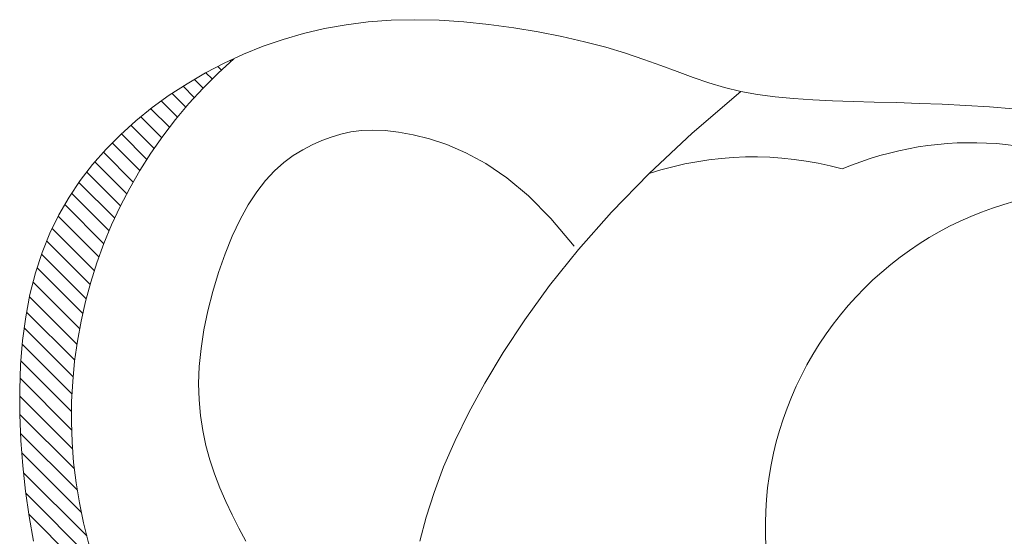
# Model space of a CAD drawing. Units: inches. Extents: x -17 to 1735, y -531 to 60.
# Tile 8 of 27: x 1734.671706 to 1734.675388, y -150.218274 to -150.216342. Entities that reach past the tile are written whole.
import ezdxf

# ---------------------------------------------------------------- set-up
doc = ezdxf.new("R2010")
doc.units = ezdxf.units.IN
doc.header["$MEASUREMENT"] = 0
doc.layers.add('A-FURN', color=242, linetype='Continuous', lineweight=18, true_color=0xcd2027)

# ---------------------------------------------------------------- blocks, each defined once
blk = doc.blocks.new('childrens_room_2')
for p, q in [((70.11022739858484, 54.15762691826097), (70.11227292050492, 54.15799201522753)), ((70.11227292050492, 54.15799201522753), (70.11437812355464, 54.15825517993511)), ((70.11437812355464, 54.15825517993511), (70.11654878333096, 54.1584144891371)), ((70.11654878333096, 54.1584144891371), (70.1187906754308, 54.15846801959418)), ((70.1187906754308, 54.15846801959418), (70.12110363943387, 54.15841577130635)), ((70.12110363943387, 54.15841577130635), (70.1234637707926, 54.15826543726729)), ((70.1234637707926, 54.15826543726729), (70.12584122900037, 54.15802663372454)), ((70.12584122900037, 54.15802663372454), (70.12820617337594, 54.15770897692567)), ((70.10629229580402, 54.15659862055185), (70.10823578225566, 54.1571618122893)), ((70.10823578225566, 54.1571618122893), (70.11022739858484, 54.15762691826097)), ((70.12820617337594, 54.15770897692567), (70.13052876347095, 54.15732208312551)), ((70.13052876347095, 54.15732208312551), (70.13277915866232, 54.15687556855704)), ((70.13277915866232, 54.15687556855704), (70.13492751844345, 54.15637904946783)), ((70.10252661037842, 54.15518567278053), (70.10439116369119, 54.15593926630248)), ((70.10439116369119, 54.15593926630248), (70.10629229580402, 54.15659862055185)), ((70.13492751844345, 54.15637904946783), (70.13694400219131, 54.15584214210543)), ((70.10069526663167, 54.15434008377491), (70.10252661037842, 54.15518567278053)), ((70.13694400219131, 54.15584214210543), (70.13880855579512, 54.1552752640768)), ((70.13880855579512, 54.1552752640768), (70.14054027072737, 54.15469203840479)), ((70.09890338942526, 54.15340602525105), (70.10069526663167, 54.15434008377491)), ((70.10042017687695, 54.15368526775131), (70.10008399876418, 54.15402144587864)), ((70.10132402636694, 54.15451022646306), (70.1012418118876, 54.15459244092057)), ((70.14054027072737, 54.15469203840479), (70.14216802503098, 54.15410688947162)), ((70.14216802503098, 54.15410688947162), (70.14372069663251, 54.15353424165227)), ((70.0971596421546, 54.15238734370217), (70.09890338942526, 54.15340602525105)), ((70.09953980340973, 54.15283683302408), (70.09894757724717, 54.15342905918663)), ((70.14372069663251, 54.15353424165227), (70.14522716345849, 54.15298851932897)), ((70.09547268815689, 54.15128788564328), (70.0971596421546, 54.15238734370217)), ((70.09784939513659, 54.1510696248792), (70.09677945811885, 54.1521395619406)), ((70.09868287063321, 54.15196495756976), (70.09785453458201, 54.15279329364278)), ((70.14522716345849, 54.15298851932897), (70.1467163034936, 54.15248414689125)), ((70.1467163034936, 54.15248414689125), (70.14821699472262, 54.15203554871408)), ((70.09385119088577, 54.15011149757487), (70.09547268815689, 54.15128788564328)), ((70.09703944531387, 54.15015076649291), (70.09573280032376, 54.15145741153395)), ((70.14975811495563, 54.1516571491797), (70.1451421334746, 54.14769204849875)), ((70.14821699472262, 54.15203554871408), (70.14975811495563, 54.1516571491797)), ((70.14975811495563, 54.1516571491797), (70.15136372933515, 54.15135888507797)), ((70.15136372933515, 54.15135888507797), (70.1530386507616, 54.1511327428729)), ((70.09625314241158, 54.14920826122255), (70.09471976205126, 54.15074164156834)), ((70.1530386507616, 54.1511327428729), (70.15478287929321, 54.15096622143614)), ((70.15478287929321, 54.15096622143614), (70.15659641487176, 54.15084681965385)), ((70.15659641487176, 54.15084681965385), (70.15847925761366, 54.15076203638313)), ((70.15847925761366, 54.15076203638313), (70.16043140746072, 54.1506993704956)), ((70.16043140746072, 54.1506993704956), (70.16245286441293, 54.15064632088473)), ((70.16245286441293, 54.15064632088473), (70.16454362852849, 54.1505903864076)), ((70.16454362852849, 54.1505903864076), (70.1667004911101, 54.15052050837989)), ((70.1667004911101, 54.15052050837989), (70.16890740884585, 54.15043139786433)), ((70.16890740884585, 54.15043139786433), (70.17114512978472, 54.15031920834593)), ((70.17114512978472, 54.15031920834593), (70.17339440191746, 54.15018009333147)), ((70.09230381367846, 54.14886202599013), (70.09385119088577, 54.15011149757487)), ((70.09549066163484, 54.1482419337903), (70.09372389020749, 54.15000870521038)), ((70.17339440191746, 54.15018009333147), (70.17563597329311, 54.15001020629865)), ((70.09083921987215, 54.14754331740408), (70.09230381367846, 54.14886202599013)), ((70.09403815080762, 54.14623682820678), (70.09183503636044, 54.14843994265396)), ((70.09475223441726, 54.1472515528207), (70.09276741435636, 54.14923637289615)), ((70.0894660729787, 54.14615921831722), (70.09083921987215, 54.14754331740408)), ((70.09334876319511, 54.14519740760301), (70.09092532506796, 54.14762084579564)), ((70.11178336607875, 54.14759831467967), (70.11086421542453, 54.14732131697241)), ((70.11273538636625, 54.14780503082005), (70.11178336607875, 54.14759831467967)), ((70.11373901793152, 54.1479339763668), (70.11273538636625, 54.14780503082005)), ((70.11481300218614, 54.14797766230771), (70.11373901793152, 54.1479339763668)), ((70.11597608065816, 54.14792859963057), (70.11481300218614, 54.14797766230771)), ((70.11724699487561, 54.14777929933046), (70.11597608065816, 54.14792859963057)), ((70.11864448630834, 54.14752227237335), (70.11724699487561, 54.14777929933046)), ((70.12018201035565, 54.14714273276189), (70.11864448630834, 54.14752227237335)), ((70.1451421334746, 54.14769204849875), (70.14106135688374, 54.14386157530538)), ((70.09268449044205, 54.14413287219071), (70.09005974111963, 54.14675762152768)), ((70.10905344989035, 54.14658249635107), (70.10814770667233, 54.14611203226235)), ((70.10995919305017, 54.1469815267032), (70.10905344989035, 54.14658249635107)), ((70.11086421542453, 54.14732131697241), (70.10995919305017, 54.1469815267032)), ((70.12185187825119, 54.14659670650002), (70.12018201035565, 54.14714273276189)), ((70.12364111515811, 54.1458329225847), (70.12185187825119, 54.14659670650002)), ((70.08819191327669, 54.14471197251845), (70.0894660729787, 54.14615921831722)), ((70.0920458231226, 54.14304273130841), (70.08921477321886, 54.14587378119762)), ((70.10814770667233, 54.14611203226235), (70.10724657681888, 54.14555400424291)), ((70.12553674612312, 54.14480011004929), (70.12364111515811, 54.1458329225847)), ((70.08701978898492, 54.14319741297226), (70.08819191327669, 54.14471197251845)), ((70.09143333015848, 54.14192641607809), (70.08840534674121, 54.14495439950991)), ((70.10635467351997, 54.14489228209863), (70.10547661008198, 54.14411073563536)), ((70.10724657681888, 54.14555400424291), (70.10635467351997, 54.14489228209863)), ((70.12752579625113, 54.14344699788347), (70.12553674612312, 54.14480011004929)), ((70.09084766650224, 54.14078327153987), (70.08763656207476, 54.14399437593823)), ((70.10547661008198, 54.14411073563536), (70.10461699986946, 54.14319323465901)), ((70.14106135688374, 54.14386157530538), (70.13747343084427, 54.14016957610733)), ((70.08595162532177, 54.14160976992429), (70.08701978898492, 54.14319741297226)), ((70.09028958256707, 54.13961254725876), (70.0868930671818, 54.14300906265856)), ((70.10461699986946, 54.14319323465901), (70.10378045607243, 54.1421236489827)), ((70.12959529076355, 54.14172231509877), (70.12752579625113, 54.14344699788347)), ((70.0897599357518, 54.13841338586502), (70.0861977416894, 54.14197557994197)), ((70.10378045607243, 54.1421236489827), (70.10297159205541, 54.14088584841232)), ((70.08498934750563, 54.13994327362019), (70.08595162532177, 54.14160976992429)), ((70.08925970423618, 54.13718480922984), (70.08554278431578, 54.14090172909931)), ((70.10297159205541, 54.14088584841232), (70.10219588603243, 54.13947195987424)), ((70.13173225464882, 54.13957479070671), (70.12959529076355, 54.14172231509877)), ((70.13747343084427, 54.14016957610733), (70.13433600107558, 54.13661989740507)), ((70.08413488075487, 54.13819215430561), (70.08498934750563, 54.13994327362019)), ((70.08879000368646, 54.13592570158511), (70.08491821285455, 54.13979749237336)), ((70.10219588603243, 54.13947195987424), (70.1014622763137, 54.13790713879865)), ((70.13392371312833, 54.13695315371882), (70.13173225464882, 54.13957479070671)), ((70.08339015022968, 54.13635064224076), (70.08413488075487, 54.13819215430561)), ((70.0883521081519, 54.1346347888961), (70.08435127355509, 54.13863562348564)), ((70.08794747544337, 54.13331061339562), (70.08382706857402, 54.13743102025768)), ((70.1014622763137, 54.13790713879865), (70.10078056617525, 54.13622479772169)), ((70.08275708114846, 54.13441296767127), (70.08339015022968, 54.13635064224076)), ((70.10078056617525, 54.13622479772169), (70.1001605587767, 54.13445834920134)), ((70.13433600107558, 54.13661989740507), (70.13160671318067, 54.13321638569908)), ((70.08757777868189, 54.13195150196992), (70.08333806351177, 54.13619121716187)), ((70.08223759867136, 54.13237336082824), (70.08275708114846, 54.13441296767127)), ((70.08724494605443, 54.13055552643931), (70.08291232872173, 54.13488814376473)), ((70.1001605587767, 54.13445834920134), (70.09961205745233, 54.13264120578827)), ((70.08695121104714, 54.12912045320848), (70.08253411449142, 54.13353754976419)), ((70.09961205745233, 54.13264120578827), (70.09914486536175, 54.13080678001865)), ((70.13160671318067, 54.13321638569908), (70.12924321276253, 54.12996288750441)), ((70.08183250507457, 54.1302298984869), (70.08223759867136, 54.13237336082824)), ((70.08669917752152, 54.12764367854691), (70.08219498356223, 54.13214787250621)), ((70.08649190364989, 54.12612214423865), (70.08192018903677, 54.13069385881539)), ((70.09914486536175, 54.13080678001865), (70.09876878583921, 54.12898848445042)), ((70.08153811028345, 54.12799604338073), (70.08183250507457, 54.1302298984869)), ((70.12924321276253, 54.12996288750441), (70.12720314548235, 54.12686324931422)), ((70.08633301384864, 54.12455222585271), (70.0816954336001, 54.12918980608669)), ((70.09876878583921, 54.12898848445042), (70.09849362210255, 54.12721973161973)), ((70.08134960133933, 54.12568910476551), (70.08153811028345, 54.12799604338073)), ((70.0862268496526, 54.12292958180336), (70.08150957671344, 54.12764685476435)), ((70.09849362210255, 54.12721973161973), (70.09832658247208, 54.1255270211463)), ((70.12720314548235, 54.12686324931422), (70.12544415705955, 54.12392131764358)), ((70.08617867804017, 54.12124894522861), (70.08137898060843, 54.12604864268946)), ((70.08126216528356, 54.1233263919043), (70.08134960133933, 54.12568910476551)), ((70.09832658247208, 54.1255270211463), (70.09826449521236, 54.12390920087495)), ((70.08619498573128, 54.11950382936487), (70.08130178595778, 54.124397029102)), ((70.0812709890993, 54.12092521403105), (70.08126216528356, 54.1233263919043)), ((70.09826449521236, 54.12390920087495), (70.09830159380682, 54.12235820569043)), ((70.12544415705955, 54.12392131764358), (70.12392790389598, 54.12113693221039)), ((70.08628390875995, 54.11768609811992), (70.08126444673283, 54.12270556015432)), ((70.09830159380682, 54.12235820569043), (70.09843211156434, 54.12086597052115)), ((70.08645588125685, 54.11578531745039), (70.08127082314925, 54.12097037552161)), ((70.08137125982788, 54.11850288041609), (70.0812709890993, 54.12092521403105)), ((70.09843211156434, 54.12086597052115), (70.0986502819101, 54.11942443025186)), ((70.12392790389598, 54.12113693221039), (70.12263208576363, 54.11849390566789)), ((70.0986502819101, 54.11942443025186), (70.09895033815295, 54.11802551979639)), ((70.08672465792509, 54.11378773255131), (70.08134369908251, 54.11916869141572)), ((70.08155816439422, 54.11607670030065), (70.08137125982788, 54.11850288041609)), ((70.12263208576363, 54.11849390566789), (70.12153841334978, 54.11597204388676)), ((70.09895033815295, 54.11802551979639), (70.09932651377633, 54.11666117404678)), ((70.08710901591579, 54.11167456635888), (70.0814622849098, 54.11732129736487)), ((70.09932651377633, 54.11666117404678), (70.09977304214729, 54.11532332792416)), ((70.08182688989794, 54.1136639829478), (70.08155816439422, 54.11607670030065)), ((70.12153841334978, 54.11597204388676), (70.1206285972253, 54.11355115273767)), ((70.08763578459505, 54.10941898947789), (70.08163087228198, 54.11542390179096)), ((70.09977304214729, 54.11532332792416), (70.10028319550796, 54.11400526050278)), ((70.10028319550796, 54.11400526050278), (70.10084640171729, 54.11270562759312)), ((70.08217230242329, 54.11128011434488), (70.08182688989794, 54.1136639829478)), ((70.08834575234098, 54.10698021353749), (70.08185483306764, 54.11347113283994)), ((70.1206285972253, 54.11355115273767), (70.11988434807748, 54.11121103807676)), ((70.10084640171729, 54.11270562759312), (70.10145112762578, 54.11142442920976)), ((70.08930673154421, 54.10429042615437), (70.08214777633432, 54.11144938138608)), ((70.08258798463388, 54.10893278750013), (70.08217230242329, 54.11128011434488)), ((70.10145112762578, 54.11142442920976), (70.10208583985107, 54.11016166533085)), ((70.11988434807748, 54.11121103807676), (70.11928737653537, 54.10893150579653)), ((70.10208583985107, 54.11016166533085), (70.10273900536006, 54.10891733597094))]:
    blk.add_line(p, q)
for centre, radius, start, end in [((70.13126567467, 54.1207976377322), 0.0450892553131211, 131.1239089098638, 210.6911252888027), ((70.17166475667503, 54.11546908731401), 0.0313149888669701, 58.27266326727306, 113.0496076004186), ((70.1509342570894, 54.11361584136324), 0.0318163256877229, 74.56117099046632, 108.0778683786329), ((70.18419688196039, 54.11024985505941), 0.0320967331381597, 82.95662561159509, 211.3772048657365)]:
    blk.add_arc(centre, radius, start, end)

msp = doc.modelspace()

# ---------------------------------------------------------------- block references
at = {"layer": 'A-FURN', "xscale": 0.0393700787401575, "yscale": 0.0393700787401575, "zscale": 0.0393700787401575}
msp.add_blockref('childrens_room_2', (1731.912600860487, -152.3485650223338), dxfattribs=at)

doc.saveas('drawing.dxf')
